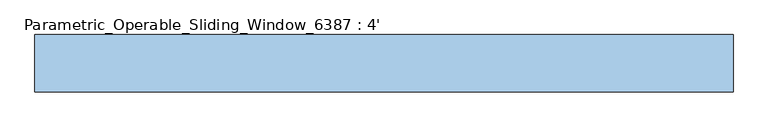
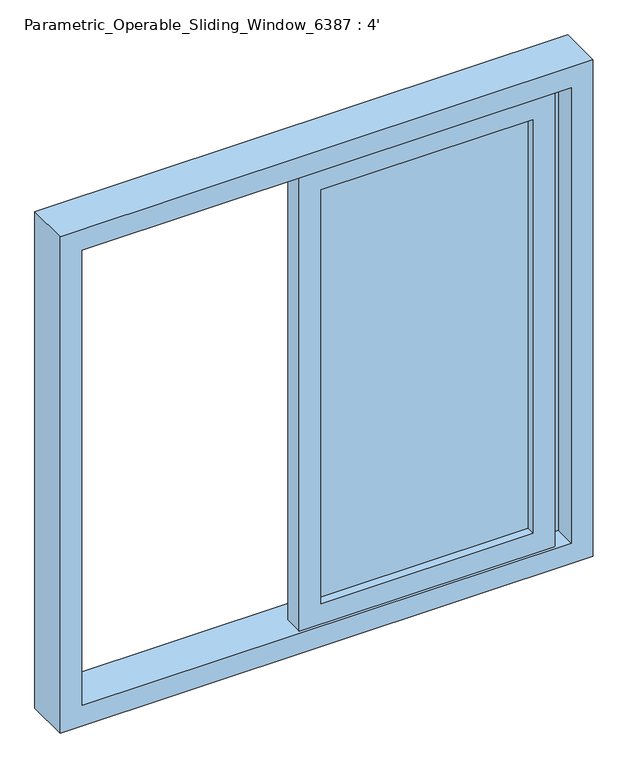
"""IFC4 building model written with IfcOpenShell, lengths in millimetres: window geometry, Parametric_Operable_Sliding_Window_6387 : 4'."""

from ifc_helpers import new_model, si_unit, frame, origin, place, context, project, spatial, polyline, outline, extrude, source, transform, mapped, element, save


def parametric_operable_sliding_window_6387_4_f716cbab(model_context):
    return source(origin(), model_context, "Body", "SweptSolid", [
        extrude(outline(polyline([(900.0, 869.6), (2100.0, 869.6), (2100.0, -349.6), (900.0, -349.6), (900.0, 869.6)]), holes=[polyline([(2050.0, -299.6), (2050.0, 819.6), (950.0, 819.6), (950.0, -299.6), (2050.0, -299.6)])]), frame((0.0, -50.0, 0.0), z_axis=(0.0, 1.0, 0.0), x_axis=(0.0, 0.0, 1.0)), (0.0, 0.0, 1.0), 100.0),
        extrude(outline(polyline([(2050.0, 235.0), (950.0, 235.0), (950.0, 819.6), (2050.0, 819.6), (2050.0, 235.0)]), holes=[polyline([(2000.0, 285.0), (2000.0, 769.6), (1000.0, 769.6), (1000.0, 285.0), (2000.0, 285.0)])]), frame((0.0, 0.0, 0.0), z_axis=(0.0, 1.0, 0.0), x_axis=(0.0, 0.0, 1.0)), (0.0, 0.0, 1.0), 45.0),
        extrude(outline(polyline([(769.6, 16.5), (285.0, 16.5), (285.0, 22.5), (769.6, 22.5), (769.6, 16.5)])), frame((0.0, 0.0, 1000.0), z_axis=(0.0, 0.0, 1.0), x_axis=(1.0, 0.0, 0.0)), (0.0, 0.0, 1.0), 1000.0),
        extrude(outline(polyline([(950.0, 200.4), (950.0, 785.0), (2050.0, 785.0), (2050.0, 200.4), (950.0, 200.4)]), holes=[polyline([(2000.0, 250.4), (2000.0, 735.0), (1000.0, 735.0), (1000.0, 250.4), (2000.0, 250.4)])]), frame((0.0, -45.0, 0.0), z_axis=(0.0, 1.0, 0.0), x_axis=(0.0, 0.0, 1.0)), (0.0, 0.0, 1.0), 45.0),
        extrude(outline(polyline([(250.4, -25.5), (250.4, -19.5), (735.0, -19.5), (735.0, -25.5), (250.4, -25.5)])), frame((0.0, 0.0, 1000.0), z_axis=(0.0, 0.0, 1.0), x_axis=(1.0, 0.0, 0.0)), (0.0, 0.0, 1.0), 1000.0),
    ])


if __name__ == "__main__":
    model = new_model("IFC4")
    model_context = context("Model", 3, world=origin())
    ifc_project = project(units=[si_unit("LENGTHUNIT", "METRE", prefix="MILLI")], contexts=[model_context])
    site = spatial("IfcSite", under=ifc_project)
    building = spatial("IfcBuilding", under=site)
    placement = place(None, origin())
    parametric_operable_sliding_window_6387_4_shape = parametric_operable_sliding_window_6387_4_f716cbab(model_context)
    element("IfcWindow", 1, ObjectType="Parametric_Operable_Sliding_Window_6387 : 4'", at=placement, inside=building, context=model_context, shape_type="MappedRepresentation", body=[
        mapped(parametric_operable_sliding_window_6387_4_shape, transform((0.0, 0.0, 0.0), x_axis=(1.0, 0.0, 0.0), y_axis=(0.0, 1.0, 0.0), z_axis=(0.0, 0.0, 1.0))),
    ])
    save(model, "model.ifc")

# Revit data of these elements
# Type "Parametric_Operable_Sliding_Window_6387 : 4'"
#   Type Mark = "62"
#   Sash Offset From Frame = 0' - 0"
#   Sash Width = 0' - 3.54331"
#   Sash Thickness = 0' - 1.9685"
#   Sash Edge Offset = 0' - 0.19685"
#   Rough Tolerance = 0' - 0.3937"
#   Rough Width = 4' - 1.33858"
#   Rough Height = 4' - 0.58268"
#   Reveal Thickness = 0' - 0.47244"
#   Panel Sash Depth = 0' - 1.77165"
#   Pane Width = 1' - 11.01575"
#   Pane Height = 3' - 7.30709"
#   Opened Pane Portion [instance default] = 1' - 7.68504"
#   Glass Thickness = 0' - 0.23622"
#   Frame Offset = 0' - 0"
#   Height = 3' - 11.24409"
#   Frame Width = 0' - 3.93701"
#   Frame Thickness = 0' - 1.9685"
#   Frame Sill = 0' - 0.98425"
#   Width = 4' - 0"
#   Default Sill Height = 2' - 11.43307"
#   Architrave Width = 0' - 2.67717"
#   Architrave Thickness = 0' - 0.47244"
#   Architrave Offset = 0' - 0.19685"
#   Show Reveal = no
#   Show Architrave = no
#   Reveal = Window Reveal
#   Glass = Window Glass
#   Frame = Window Frame
#   Architrave = Window Architrave
#   Wall Closure = (empty or 0)
#   Assembly Code = ""
# Element 1 (IfcWindow, "Parametric_Operable_Sliding_Window_6387 : 4'")
#   Materials on its faces: "Window Frame", "Window Glass"
# Materials
#   "Window Reveal": colour RGB 255 255 255, transparency 0
#   "Window Glass": colour RGB 0 0 255, transparency 0.75
#   "Window Frame": colour RGB 249 249 249, transparency 0, Keynote = "L10", Cost = 0
#   "Window Architrave": colour RGB 255 255 255, transparency 0
